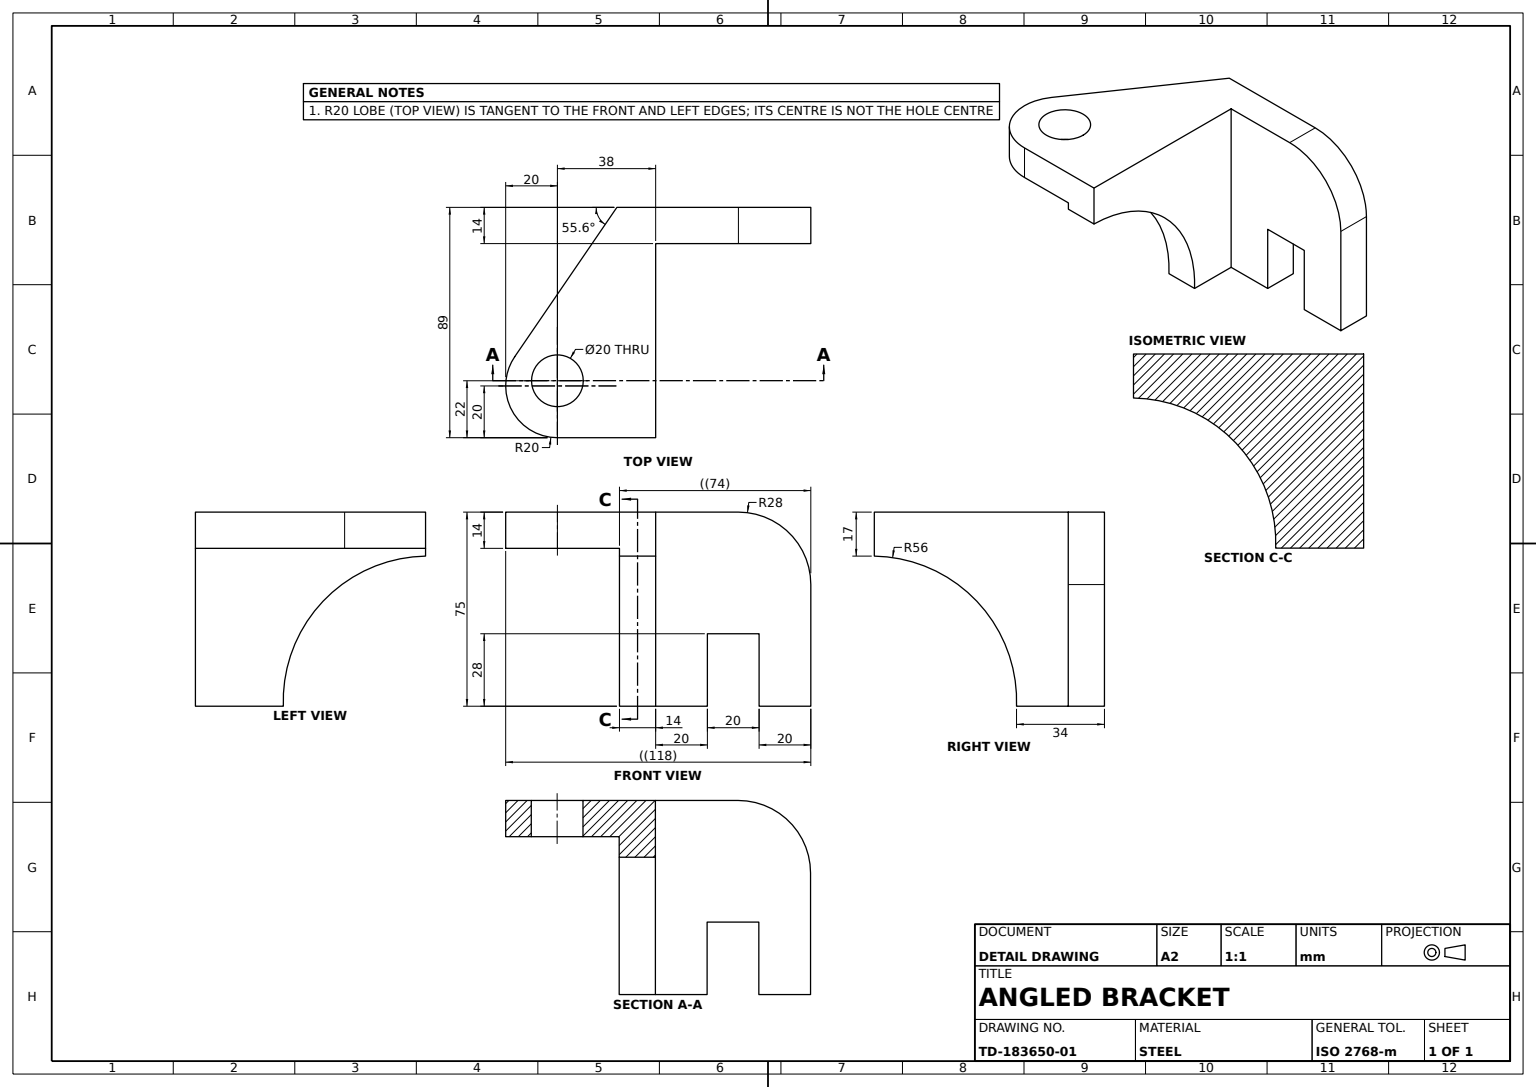
SolidWorks part; units mm, degrees
material "Plain Carbon Steel"
ref_plane "Front Plane" through (0, 0, 0) normal (0, 0, 1) x (1, 0, 0)
ref_plane "Top Plane" through (0, 0, 0) normal (0, 1, 0) x (1, 0, 0)
ref_plane "Right Plane" through (0, 0, 0) normal (1, 0, 0) x (0, 0, -1)
sketch "Base Plate Sketch" plane through (0, 0, 0) normal (0, 0, 1) x (1, 0, 0)
  line L0 (1, 0) -> (1, 75)
  line L1 (1, 75) -> (75, 75)
  line L2 (75, 75) -> (75, 0)
  line L3 (75, 0) -> (55, 0)
  line L4 (55, 0) -> (55, 28)
  line L5 (55, 28) -> (35, 28)
  line L6 (35, 28) -> (35, 0)
  line L7 (35, 0) -> (1, 0)
  line L8 (0, 0) -> (75, 0) construction
  dimension "D1" = 75
  dimension "D2" = 74
  dimension "D3" = 20
  dimension "D4" = 20
  dimension "D5" = 28
  dimension "D6" = 1
extrude "Base Plate 14mm" add sketch "Base Plate Sketch" along normal blind 14
sketch "Upright Web Sketch" plane through (0, 0, 0) normal (1, 0, 0) x (0, 0, -1)
  line L0 (-14, 75) -> (-89, 75)
  line L1 (-89, 75) -> (-89, 58)
  line L2 (-14, 0) -> (-34, 0)
  line L7 (0, 0) -> (0, 75)
  line L8 (0, 75) -> (-14, 75)
  line L9 (-14, 75) -> (-14, 0)
  line L10 (-14, 0) -> (0, 0)
  line L13 (-14, 75) -> (-14, 0)
  arc A1 (-89, 58) -> (-34, 0) centre (-89.964, 2.0083) cw
  dimension "D4" = 56
  dimension "D1" = 75
  dimension "D2" = 17
  dimension "D3" = 20
  dimension "D5" = 0
extrude "Upright Web 14mm" add sketch "Upright Web Sketch" along normal blind 14 from offset 1
sketch "Side Lug Sketch" plane through (0, 75, 0) normal (0, 1, 0) x (1, 0, 0)
  line L0 (1, -89) -> (-23, -89)
  line L2 (-39.5031, -57.7019) -> (0, 0)
  line L3 (15, -14) -> (15, -89) construction
  line L5 (15, -89) -> (1, -89) construction
  line L8 (0, 0) -> (1, 0)
  line L9 (1, 0) -> (1, -89)
  circle A0 centre (-23, -67) radius 10
  arc A5 (-39.5031, -57.7019) -> (-23, -89) centre (-23, -69) ccw
  dimension "D3" = 20
  dimension "D4" = 20
  dimension "D1" = 22
  dimension "D2" = 38
  dimension "D5" = 38
extrude "Side Lug 14mm" add sketch "Side Lug Sketch" against normal blind 14
fillet "Corner Round R28" radius 28 1 edges at (75, 75, 7)
